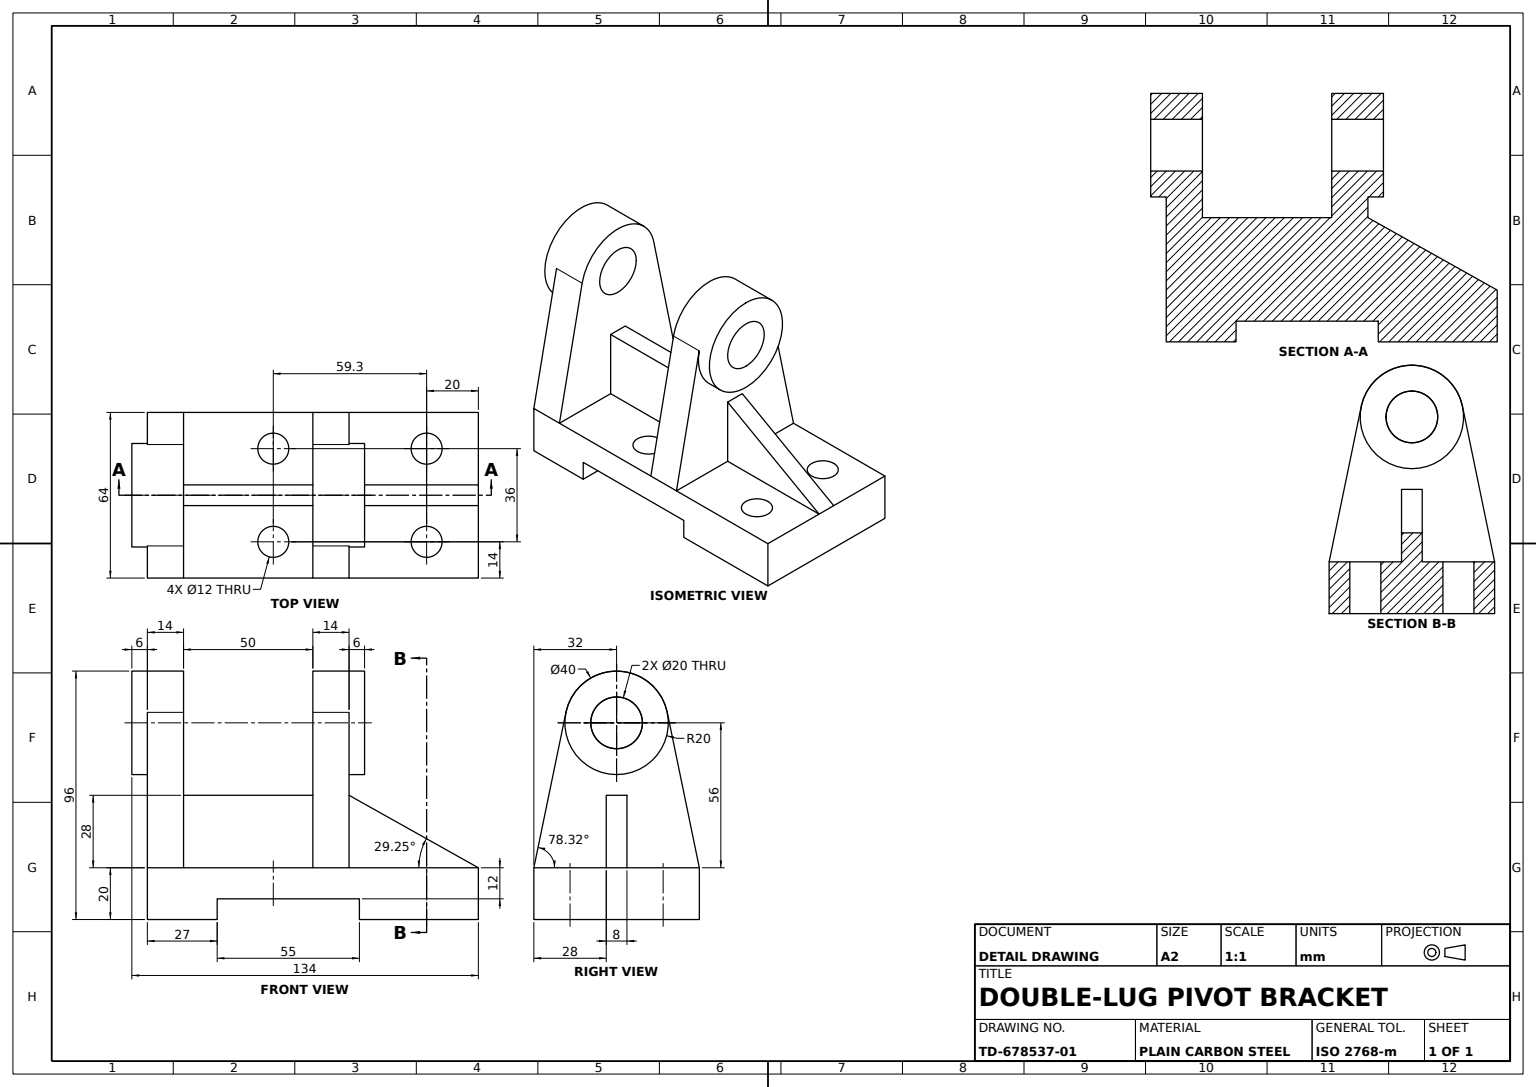
SolidWorks part; units mm, degrees
material "Plain Carbon Steel"
ref_plane "Front Plane" through (0, 0, 0) normal (0, 0, 1) x (1, 0, 0)
ref_plane "Top Plane" through (0, 0, 0) normal (0, 1, 0) x (1, 0, 0)
ref_plane "Right Plane" through (0, 0, 0) normal (1, 0, 0) x (0, 0, -1)
sketch "Base Plate Profile Sketch" plane through (0, 0, 0) normal (0, 0, 1) x (1, 0, 0)
  line L0 (0, 0) -> (27, 0)
  line L1 (27, 0) -> (82, 0)
  line L2 (82, 0) -> (128, 0)
  line L3 (128, 0) -> (128, -20)
  line L4 (128, -20) -> (82, -20)
  line L5 (0, 0) -> (0, -20)
  line L6 (0, -20) -> (27, -20)
  line L8 (27, -20) -> (27, -12)
  line L9 (27, -12) -> (82, -12)
  line L10 (82, -12) -> (82, -20)
  dimension "D1" = 27
  dimension "D2" = 55
  dimension "D3" = 46
  dimension "D4" = 20
  dimension "D5" = 46
  dimension "D6" = 20
  dimension "D7" = 27
  dimension "D8" = 12
extrude "Base Plate" add sketch "Base Plate Profile Sketch" against normal blind 64
sketch "Clevis Lug 1 Sketch" plane through (0, 0, 0) normal (-1, 0, 0) x (0, 0, 1)
  line L0 (-32, 0) -> (-32, 56)
  line L1 (-64, 0) -> (0, 0) construction
  line L2 (-64, 0) -> (0, 0)
  line L3 (0, 0) -> (-12.4142, 60.0491)
  line L4 (-64, 0) -> (-51.5858, 60.0491)
  arc A0 (-12.4142, 60.0491) -> (-51.5858, 60.0491) centre (-32, 56) ccw
  dimension "D2" = 40
  dimension "D1" = 56
extrude "Clevis Lug 1" add sketch "Clevis Lug 1 Sketch" against normal blind 14
sketch "Lug 1 Hub Sketch" plane through (0, 0, 0) normal (-1, 0, 0) x (0, 0, 1)
  circle A0 centre (-32, 56) radius 20
  dimension "D1" = 40
extrude "Lug 1 Hub Boss Ø40" add sketch "Lug 1 Hub Sketch" along normal blind 6
sketch "Lug 1 Pin Bore Sketch" plane through (-6, 0, 0) normal (-1, 0, 0) x (0, 0, 1)
  circle A0 centre (-32, 56) radius 10
  dimension "D1" = 20
extrude "Lug 1 Pin Bore Ø20" cut sketch "Lug 1 Pin Bore Sketch" against normal blind 30
sketch "Web Block Sketch" plane through (0, 0, 0) normal (0, 0, 1) x (1, 0, 0)
  line L0 (14, 0) -> (14, 28)
  line L1 (14, 0) -> (14, 60.0491) construction
  line L2 (14, 28) -> (64, 28)
  line L3 (64, 28) -> (64, 0)
  line L4 (128, 0) -> (14, 0) construction
  line L5 (64, 0) -> (14, 0)
  dimension "D1" = 28
  dimension "D2" = 50
extrude "Web Block" add sketch "Web Block Sketch" against normal blind 64
sketch "Web Trim Cut 1 Sketch" plane through (0, 0, 0) normal (0, 0, 1) x (1, 0, 0)
  line L0 (14, 28) -> (14, 0)
  line L1 (14, 0) -> (64, 0)
  line L2 (64, 0) -> (64, 28)
  line L3 (64, 28) -> (14, 28)
extrude "Web Trim Cut 1" cut sketch "Web Trim Cut 1 Sketch" against normal blind 28
sketch "Web Trim Cut 2 Sketch" plane through (0, 0, -64) normal (0, 0, -1) x (-1, 0, 0)
  line L0 (-64, 28) -> (-64, 0)
  line L1 (-64, 0) -> (-14, 0)
  line L2 (-14, 0) -> (-14, 28)
  line L3 (-14, 28) -> (-64, 28)
extrude "Web Trim Cut 2" cut sketch "Web Trim Cut 2 Sketch" against normal blind 28
sketch "Clevis Lug 2 Sketch" plane through (64, 0, 0) normal (1, 0, 0) x (0, 0, -1)
  line L0 (0, 0) -> (12.4142, 60.0491)
  line L1 (64, 0) -> (51.5858, 60.0491)
  line L2 (0, 0) -> (64, 0)
  arc A0 (51.5858, 60.0491) -> (12.4142, 60.0491) centre (32, 56) ccw
  dimension "D1" = 40
extrude "Clevis Lug 2" add sketch "Clevis Lug 2 Sketch" along normal blind 14
sketch "Lug 2 Hub Sketch" plane through (78, 0, 0) normal (1, 0, 0) x (0, 0, -1)
  circle A0 centre (32, 56) radius 20
  dimension "D1" = 40
extrude "Lug 2 Hub Boss Ø40" add sketch "Lug 2 Hub Sketch" along normal blind 6
sketch "Lug 2 Pin Bore Sketch" plane through (84, 0, 0) normal (1, 0, 0) x (0, 0, -1)
  circle A0 centre (32, 56) radius 10
  dimension "D1" = 20
extrude "Lug 2 Pin Bore Ø20" cut sketch "Lug 2 Pin Bore Sketch" against normal blind 30
sketch "Gusset Block Sketch" plane through (0, 0, 0) normal (0, 0, 1) x (1, 0, 0)
  line L0 (78, 0) -> (78, 28)
  line L1 (78, 60.0491) -> (78, 0) construction
  line L2 (78, 28) -> (128, 0)
  line L3 (128, 0) -> (78, 0)
  dimension "D1" = 28
extrude "Gusset Block" add sketch "Gusset Block Sketch" against normal blind 64
sketch "Gusset Trim Cut 1 Sketch" plane through (0, 0, 0) normal (0, 0, 1) x (1, 0, 0)
  line L0 (78, 28) -> (78, 0)
  line L1 (78, 0) -> (128, 0)
  line L2 (128, 0) -> (78, 28)
extrude "Gusset Trim Cut 1" cut sketch "Gusset Trim Cut 1 Sketch" against normal blind 28
sketch "Gusset Trim Cut 2 Sketch" plane through (0, 0, -64) normal (0, 0, -1) x (-1, 0, 0)
  line L0 (-128, 0) -> (-78, 0)
  line L1 (-78, 0) -> (-78, 28)
  line L2 (-78, 28) -> (-128, 0)
extrude "Gusset Trim Cut 2" cut sketch "Gusset Trim Cut 2 Sketch" against normal blind 28
sketch "Mounting Holes Sketch" plane through (0, 0, 0) normal (0, 1, 0) x (1, 0, 0)
  line L0 (128, 28) -> (128, 0) construction
  line L1 (128, 64) -> (128, 36) construction
  line L2 (128, 36) -> (128, 28) construction
  line L3 (84, 32) -> (128, 32)
  line L4 (84, 12) -> (84, 52) construction
  line L5 (14, 32) -> (64, 32)
  line L6 (14, 28) -> (14, 36) construction
  line L7 (64, 51.5858) -> (64, 12.4142) construction
  circle A0 centre (48.7, 14) radius 6
  circle A1 centre (48.7, 50) radius 6
  circle A2 centre (108, 50) radius 6
  circle A3 centre (108, 14) radius 6
  dimension "D1" = 12
  dimension "D2" = 12
  dimension "D3" = 12
  dimension "D4" = 12
  dimension "D5" = 20
  dimension "D6" = 20
  dimension "D7" = 18
  dimension "D8" = 18
  dimension "D9" = 59.3
  dimension "D10" = 18
  dimension "D11" = 59.3
  dimension "D12" = 18
extrude "Mounting Holes Ø12" cut sketch "Mounting Holes Sketch" against normal blind 28 contours A1 | A2 | A3 | A0
